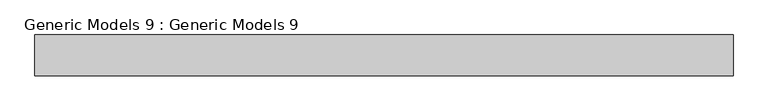
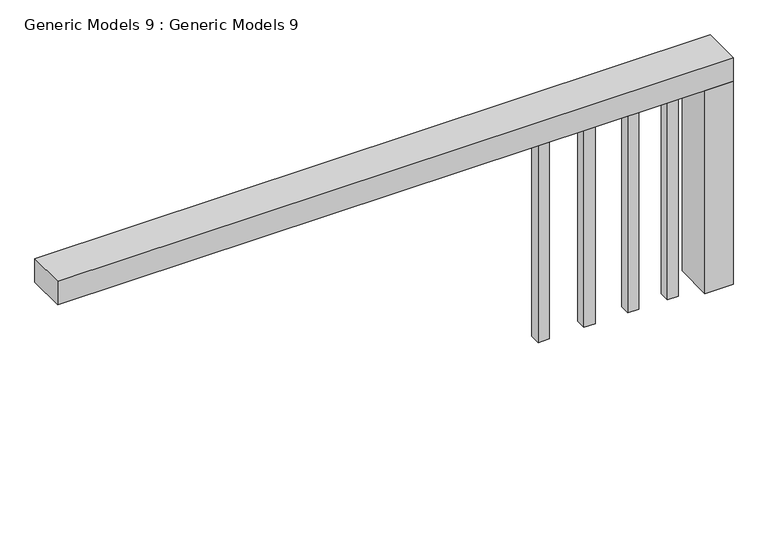
"""IFC4 building model written with IfcOpenShell, lengths in millimetres: proxy geometry, Generic Models 9 : Generic Models 9."""

from ifc_helpers import new_model, si_unit, frame, origin, place, context, project, spatial, polyline, outline, extrude, source, transform, mapped, element, save


def generic_models_9_generic_models_9_faf0bcb1(model_context):
    return source(origin(), model_context, "Body", "SweptSolid", [
        extrude(outline(polyline([(9126.0713802, -3879.5702445), (9126.0713802, -4009.874389), (8990.8108478, -4009.874389), (8990.8108478, -3879.5702445), (9126.0713802, -3879.5702445)])), frame((0.0, 0.0, 5308.6), z_axis=(0.0, 0.0, 1.0), x_axis=(1.0, 0.0, 0.0)), (0.0, 0.0, 1.0), 2616.2),
        extrude(outline(polyline([(8643.4713802, -3879.5702445), (8643.4713802, -4009.874389), (8508.2108478, -4009.874389), (8508.2108478, -3879.5702445), (8643.4713802, -3879.5702445)])), frame((0.0, 0.0, 5308.6), z_axis=(0.0, 0.0, 1.0), x_axis=(1.0, 0.0, 0.0)), (0.0, 0.0, 1.0), 2616.2),
        extrude(outline(polyline([(8110.0713802, -3879.5702445), (8110.0713802, -4009.874389), (7974.8108478, -4009.874389), (7974.8108478, -3879.5702445), (8110.0713802, -3879.5702445)])), frame((0.0, 0.0, 5308.6), z_axis=(0.0, 0.0, 1.0), x_axis=(1.0, 0.0, 0.0)), (0.0, 0.0, 1.0), 2616.2),
        extrude(outline(polyline([(7551.2713802, -3879.5702445), (7551.2713802, -4009.874389), (7416.0108478, -4009.874389), (7416.0108478, -3879.5702445), (7551.2713802, -3879.5702445)])), frame((0.0, 0.0, 5308.6), z_axis=(0.0, 0.0, 1.0), x_axis=(1.0, 0.0, 0.0)), (0.0, 0.0, 1.0), 2616.2),
        extrude(outline(polyline([(9733.554407, -3629.4798155), (9733.554407, -4111.474389), (9390.3869797, -4111.474389), (9390.3869797, -3629.4798155), (9733.554407, -3629.4798155)])), frame((0.0, 0.0, 5308.6), z_axis=(0.0, 0.0, 1.0), x_axis=(1.0, 0.0, 0.0)), (0.0, 0.0, 1.0), 2616.2),
        extrude(outline(polyline([(9733.554407, -3629.4798155), (9733.554407, -4111.474389), (1503.954407, -4111.474389), (1503.954407, -3629.4798155), (9733.554407, -3629.4798155)])), frame((0.0, 0.0, 7924.8), z_axis=(0.0, 0.0, 1.0), x_axis=(1.0, 0.0, 0.0)), (0.0, 0.0, 1.0), 304.8),
    ])


if __name__ == "__main__":
    model = new_model("IFC4")
    model_context = context("Model", 3, world=origin())
    ifc_project = project(units=[si_unit("LENGTHUNIT", "METRE", prefix="MILLI")], contexts=[model_context])
    site = spatial("IfcSite", under=ifc_project)
    building = spatial("IfcBuilding", under=site)
    placement = place(None, origin())
    generic_models_9_generic_models_9_shape = generic_models_9_generic_models_9_faf0bcb1(model_context)
    element("IfcBuildingElementProxy", 1, Name="Generic Models 9 : Generic Models 9", ObjectType="Generic Models 9 : Generic Models 9", at=placement, inside=building, context=model_context, shape_type="MappedRepresentation", body=[
        mapped(generic_models_9_generic_models_9_shape, transform((0.0, 0.0, 0.0), x_axis=(1.0, 0.0, 0.0), y_axis=(0.0, 1.0, 0.0), z_axis=(0.0, 0.0, 1.0))),
    ])
    save(model, "model.ifc")

# Revit data of these elements
# Element 1 (IfcBuildingElementProxy, "Generic Models 9 : Generic Models 9")
#   Materials on its faces: "TOP HORZ"
# Materials
#   "TOP HORZ": class "Generic", colour RGB 120 120 120, transparency 0, Cost = 0
